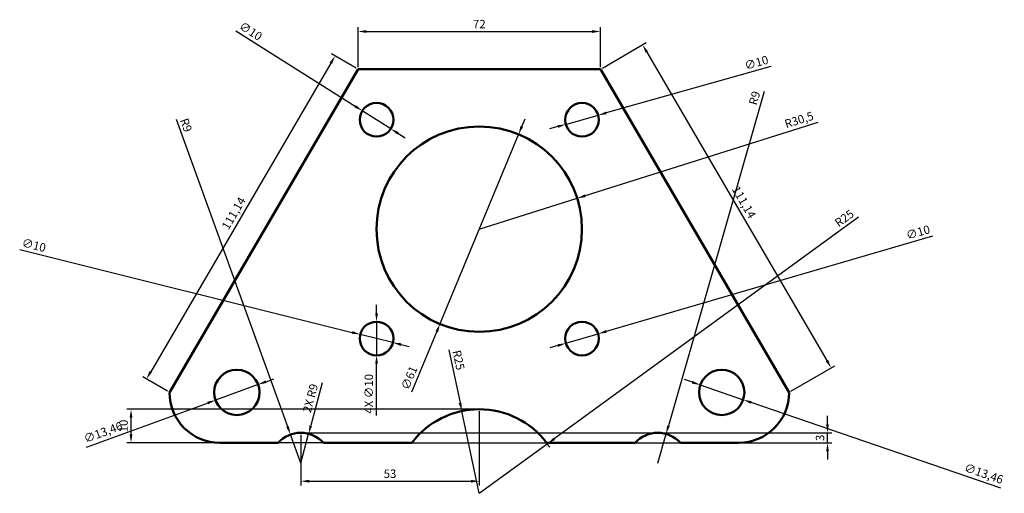
# Model space of a CAD drawing. Units: millimetres. Extents: x 120 to 412, y 203 to 344.
import ezdxf

# ---------------------------------------------------------------- set-up
doc = ezdxf.new("R2010")
doc.units = ezdxf.units.MM
doc.layers.add('M-DIMS', color=2, linetype='Continuous', lineweight=25)
doc.layers.add('M-OUTL', color=7, linetype='Continuous', lineweight=50)
doc.styles.get("Standard").update_dxf_attribs({"font": 'arial.ttf'})
doc.dimstyles.new('ISO-25', dxfattribs={"dimtxt": 2.5, "dimasz": 2.5, "dimexe": 1.25, "dimexo": 0.625, "dimtad": 1, "dimtxsty": 'Standard', "dimcen": 2.5, "dimadec": 0, "dimazin": 0, "dimtfac": 1, "dimtmove": 0, "dimatfit": 3, "dimfxl": 1, "dimarcsym": 0})

# ---------------------------------------------------------------- blocks, each defined once
blk = doc.blocks.new('*D1')
at = {"layer": 'Defpoints', "color": 0, "transparency": 16777216}
for p in [(292.1, 328.85), (360.58, 240.13), (348.1, 232.85)]:
    blk.add_point(p, dxfattribs=at)
at = {"layer": 'M-DIMS', "color": 0, "lineweight": -2, "transparency": 16777216}
for p, q in [((292.64, 329.16), (305.66, 336.76)), ((305.84, 333.97), (359.32, 242.29)), ((348.64, 233.16), (361.66, 240.76))]:
    blk.add_line(p, q, dxfattribs=at)
at = {"layer": 'M-DIMS', "color": 0, "transparency": 16777216}
for points in [[(306.2, 334.18), (305.48, 333.76), (304.58, 336.13)], [(359.68, 242.5), (358.96, 242.08), (360.58, 240.13)]]:
    blk.add_solid(points, dxfattribs=at)
at = {"layer": 'M-DIMS', "color": 0, "transparency": 16777216, "insert": (334.42, 289.2), "char_height": 2.5, "attachment_point": 5, "rotation": 300.2564}
blk.add_mtext('111,14', dxfattribs=at)
blk = doc.blocks.new('*D2')
at = {"layer": 'Defpoints', "color": 0, "transparency": 16777216}
for p in [(292.1, 340.07), (220.1, 328.85), (292.1, 328.85)]:
    blk.add_point(p, dxfattribs=at)
at = {"layer": 'M-DIMS', "color": 0, "lineweight": -2, "transparency": 16777216}
for p, q in [((220.1, 329.47), (220.1, 341.32)), ((222.6, 340.07), (289.6, 340.07)), ((292.1, 329.47), (292.1, 341.32))]:
    blk.add_line(p, q, dxfattribs=at)
at = {"layer": 'M-DIMS', "color": 0, "transparency": 16777216}
for points in [[(222.6, 340.49), (222.6, 339.65), (220.1, 340.07)], [(289.6, 340.49), (289.6, 339.65), (292.1, 340.07)]]:
    blk.add_solid(points, dxfattribs=at)
at = {"layer": 'M-DIMS', "color": 0, "transparency": 16777216, "insert": (256.1, 341.95), "char_height": 2.5, "attachment_point": 5}
blk.add_mtext('72', dxfattribs=at)
blk = doc.blocks.new('*D3')
at = {"layer": 'Defpoints', "color": 0, "transparency": 16777216}
for p in [(220.1, 328.85), (157.28, 236.82), (164.1, 232.85)]:
    blk.add_point(p, dxfattribs=at)
at = {"layer": 'M-DIMS', "color": 0, "lineweight": -2, "transparency": 16777216}
for p, q in [((219.56, 329.16), (212.2, 333.45)), ((212.02, 330.66), (158.54, 238.98)), ((163.56, 233.16), (156.2, 237.45))]:
    blk.add_line(p, q, dxfattribs=at)
at = {"layer": 'M-DIMS', "color": 0, "transparency": 16777216}
for points in [[(211.66, 330.87), (212.38, 330.45), (213.28, 332.82)], [(158.18, 239.19), (158.9, 238.77), (157.28, 236.82)]]:
    blk.add_solid(points, dxfattribs=at)
at = {"layer": 'M-DIMS', "color": 0, "transparency": 16777216, "insert": (183.45, 285.89), "char_height": 2.5, "attachment_point": 5, "rotation": 59.7436}
blk.add_mtext('111,14', dxfattribs=at)
blk = doc.blocks.new('*D4')
at = {"layer": 'Defpoints', "color": 0, "transparency": 16777216}
for p in [(200.03, 220.31), (203.1, 211.85)]:
    blk.add_point(p, dxfattribs=at)
at = {"layer": 'M-DIMS', "color": 0, "lineweight": -2, "transparency": 16777216}
for p, q in [((166.06, 313.98), (199.18, 222.66)), ((203.1, 211.85), (200.03, 220.31))]:
    blk.add_line(p, q, dxfattribs=at)
at = {"layer": 'M-DIMS', "color": 0, "transparency": 16777216}
blk.add_solid([(199.57, 222.8), (198.79, 222.52), (200.03, 220.31)], dxfattribs=at)
at = {"layer": 'M-DIMS', "color": 0, "transparency": 16777216, "insert": (168.75, 312.14), "char_height": 2.5, "attachment_point": 5, "rotation": 289.9316}
blk.add_mtext('R9', dxfattribs=at)
blk = doc.blocks.new('*D5')
at = {"layer": 'Defpoints', "color": 0, "transparency": 16777216}
for p in [(311.57, 220.5), (309.1, 211.85)]:
    blk.add_point(p, dxfattribs=at)
at = {"layer": 'M-DIMS', "color": 0, "lineweight": -2, "transparency": 16777216}
for p, q in [((340.7, 322.23), (312.26, 222.9)), ((309.1, 211.85), (311.57, 220.5))]:
    blk.add_line(p, q, dxfattribs=at)
at = {"layer": 'M-DIMS', "color": 0, "transparency": 16777216}
blk.add_solid([(311.86, 223.02), (312.66, 222.79), (311.57, 220.5)], dxfattribs=at)
at = {"layer": 'M-DIMS', "color": 0, "transparency": 16777216, "insert": (338.14, 320.21), "char_height": 2.5, "attachment_point": 5, "rotation": 74.0249}
blk.add_mtext('R9', dxfattribs=at)
blk = doc.blocks.new('*D6')
at = {"layer": 'Defpoints', "color": 0, "transparency": 16777216}
for p in [(276.3, 217.57), (256.1, 202.85)]:
    blk.add_point(p, dxfattribs=at)
at = {"layer": 'M-DIMS', "color": 0, "lineweight": -2, "transparency": 16777216}
for p, q in [((368.71, 284.93), (278.32, 219.05)), ((256.1, 202.85), (276.3, 217.57))]:
    blk.add_line(p, q, dxfattribs=at)
blk.add_arc((256.1, 202.85), 25, 33.2231, 36.8699, dxfattribs=at)
at = {"layer": 'M-DIMS', "color": 0, "transparency": 16777216}
blk.add_solid([(278.08, 219.38), (278.57, 218.71), (276.3, 217.57)], dxfattribs=at)
at = {"layer": 'M-DIMS', "color": 0, "transparency": 16777216, "insert": (364.67, 284.34), "char_height": 2.5, "attachment_point": 5, "rotation": 36.0879}
blk.add_mtext('R25', dxfattribs=at)
blk = doc.blocks.new('*D7')
at = {"layer": 'Defpoints', "color": 0, "transparency": 16777216}
for p in [(285.19, 290.51), (256.1, 281.35)]:
    blk.add_point(p, dxfattribs=at)
at = {"layer": 'M-DIMS', "color": 0, "lineweight": -2, "transparency": 16777216}
for p, q in [((356.64, 313.02), (287.57, 291.26)), ((256.1, 281.35), (285.19, 290.51))]:
    blk.add_line(p, q, dxfattribs=at)
at = {"layer": 'M-DIMS', "color": 0, "transparency": 16777216}
blk.add_solid([(287.45, 291.66), (287.7, 290.87), (285.19, 290.51)], dxfattribs=at)
at = {"layer": 'M-DIMS', "color": 0, "transparency": 16777216, "insert": (351.15, 313.52), "char_height": 2.5, "attachment_point": 5, "rotation": 17.4843}
blk.add_mtext('R30,5', dxfattribs=at)
blk = doc.blocks.new('*D8')
at = {"layer": 'Defpoints', "color": 0, "transparency": 16777216}
for p in [(291.41, 315.2), (281.78, 312.49)]:
    blk.add_point(p, dxfattribs=at)
at = {"layer": 'M-DIMS', "color": 0, "lineweight": -2, "transparency": 16777216}
for p, q in [((342.63, 329.63), (293.82, 315.88)), ((281.78, 312.49), (291.41, 315.2)), ((279.38, 311.81), (276.97, 311.14))]:
    blk.add_line(p, q, dxfattribs=at)
at = {"layer": 'M-DIMS', "color": 0, "transparency": 16777216}
for points in [[(293.7, 316.28), (293.93, 315.48), (291.41, 315.2)], [(279.27, 312.22), (279.49, 311.41), (281.78, 312.49)]]:
    blk.add_solid(points, dxfattribs=at)
at = {"layer": 'M-DIMS', "color": 0, "transparency": 16777216, "insert": (338.47, 330.51), "char_height": 2.5, "attachment_point": 5, "rotation": 15.7318}
blk.add_mtext('∅10', dxfattribs=at)
blk = doc.blocks.new('*D9')
at = {"layer": 'Defpoints', "color": 0, "transparency": 16777216}
for p in [(221.37, 316.52), (229.82, 311.18)]:
    blk.add_point(p, dxfattribs=at)
at = {"layer": 'M-DIMS', "color": 0, "lineweight": -2, "transparency": 16777216}
for p, q in [((183.8, 340.27), (219.26, 317.86)), ((229.82, 311.18), (221.37, 316.52)), ((231.94, 309.84), (234.05, 308.5))]:
    blk.add_line(p, q, dxfattribs=at)
at = {"layer": 'M-DIMS', "color": 0, "transparency": 16777216}
for points in [[(219.48, 318.21), (219.04, 317.5), (221.37, 316.52)], [(232.16, 310.19), (231.71, 309.49), (229.82, 311.18)]]:
    blk.add_solid(points, dxfattribs=at)
at = {"layer": 'M-DIMS', "color": 0, "transparency": 16777216, "insert": (188.05, 339.92), "char_height": 2.5, "attachment_point": 5, "rotation": 327.6988}
blk.add_mtext('∅10', dxfattribs=at)
blk = doc.blocks.new('*D10')
at = {"layer": 'Defpoints', "color": 0, "transparency": 16777216}
for p in [(220.75, 250.06), (230.45, 247.64)]:
    blk.add_point(p, dxfattribs=at)
at = {"layer": 'M-DIMS', "color": 0, "lineweight": -2, "transparency": 16777216}
for p, q in [((119.63, 275.27), (218.32, 250.66)), ((230.45, 247.64), (220.75, 250.06)), ((232.87, 247.03), (235.3, 246.43))]:
    blk.add_line(p, q, dxfattribs=at)
at = {"layer": 'M-DIMS', "color": 0, "transparency": 16777216}
for points in [[(218.42, 251.07), (218.22, 250.26), (220.75, 250.06)], [(232.98, 247.44), (232.77, 246.63), (230.45, 247.64)]]:
    blk.add_solid(points, dxfattribs=at)
at = {"layer": 'M-DIMS', "color": 0, "transparency": 16777216, "insert": (123.77, 276.27), "char_height": 2.5, "attachment_point": 5, "rotation": 345.9971}
blk.add_mtext('∅10', dxfattribs=at)
blk = doc.blocks.new('*D11')
at = {"layer": 'Defpoints', "color": 0, "transparency": 16777216}
for p in [(291.4, 250.25), (281.8, 247.44)]:
    blk.add_point(p, dxfattribs=at)
at = {"layer": 'M-DIMS', "color": 0, "lineweight": -2, "transparency": 16777216}
for p, q in [((390.64, 279.28), (293.8, 250.95)), ((281.8, 247.44), (291.4, 250.25)), ((279.4, 246.74), (277, 246.04))]:
    blk.add_line(p, q, dxfattribs=at)
at = {"layer": 'M-DIMS', "color": 0, "transparency": 16777216}
for points in [[(293.68, 251.35), (293.91, 250.55), (291.4, 250.25)], [(279.28, 247.14), (279.52, 246.34), (281.8, 247.44)]]:
    blk.add_solid(points, dxfattribs=at)
at = {"layer": 'M-DIMS', "color": 0, "transparency": 16777216, "insert": (386.47, 280.11), "char_height": 2.5, "attachment_point": 5, "rotation": 16.3027}
blk.add_mtext('∅10', dxfattribs=at)
blk = doc.blocks.new('*D12')
at = {"layer": 'Defpoints', "color": 0, "transparency": 16777216}
for p in [(321.73, 235.04), (334.46, 230.66)]:
    blk.add_point(p, dxfattribs=at)
at = {"layer": 'M-DIMS', "color": 0, "lineweight": -2, "transparency": 16777216}
for p, q in [((319.37, 235.85), (317.01, 236.66)), ((321.73, 235.04), (334.46, 230.66)), ((410.98, 204.35), (336.82, 229.85))]:
    blk.add_line(p, q, dxfattribs=at)
at = {"layer": 'M-DIMS', "color": 0, "transparency": 16777216}
for points in [[(319.51, 236.24), (319.23, 235.45), (321.73, 235.04)], [(336.96, 230.24), (336.69, 229.45), (334.46, 230.66)]]:
    blk.add_solid(points, dxfattribs=at)
at = {"layer": 'M-DIMS', "color": 0, "transparency": 16777216, "insert": (405.82, 208.42), "char_height": 2.5, "attachment_point": 5, "rotation": 341.0278}
blk.add_mtext('∅13,46', dxfattribs=at)
blk = doc.blocks.new('*D13')
at = {"layer": 'Defpoints', "color": 0, "transparency": 16777216}
for p in [(190.42, 235.16), (177.78, 230.54)]:
    blk.add_point(p, dxfattribs=at)
at = {"layer": 'M-DIMS', "color": 0, "lineweight": -2, "transparency": 16777216}
for p, q in [((192.77, 236.01), (195.11, 236.87)), ((190.42, 235.16), (177.78, 230.54)), ((139.42, 216.54), (175.43, 229.68))]:
    blk.add_line(p, q, dxfattribs=at)
at = {"layer": 'M-DIMS', "color": 0, "transparency": 16777216}
for points in [[(192.62, 236.4), (192.91, 235.62), (190.42, 235.16)], [(175.29, 230.07), (175.57, 229.29), (177.78, 230.54)]]:
    blk.add_solid(points, dxfattribs=at)
at = {"layer": 'M-DIMS', "color": 0, "transparency": 16777216, "insert": (144.5, 220.7), "char_height": 2.5, "attachment_point": 5, "rotation": 20.0551}
blk.add_mtext('∅13,46', dxfattribs=at)
blk = doc.blocks.new('MOUNT-HOLE-D10')
blk.add_circle((5, 5), 5)
blk = doc.blocks.new('FLANGE-MOUNT-HOLE')
blk.add_circle((6.73, 6.73), 6.73)
blk = doc.blocks.new('*D16')
at = {"layer": 'Defpoints', "color": 0, "transparency": 16777216}
for p in [(203.1, 220.85), (359.5, 220.85), (209.81, 217.85)]:
    blk.add_point(p, dxfattribs=at)
at = {"layer": 'M-DIMS', "color": 0, "lineweight": -2, "transparency": 16777216}
for p, q in [((359.5, 223.35), (359.5, 225.85)), ((203.72, 220.85), (360.75, 220.85)), ((359.5, 217.85), (359.5, 220.85)), ((210.43, 217.85), (360.75, 217.85)), ((359.5, 215.35), (359.5, 212.85))]:
    blk.add_line(p, q, dxfattribs=at)
at = {"layer": 'M-DIMS', "color": 0, "transparency": 16777216}
for points in [[(359.08, 223.35), (359.91, 223.35), (359.5, 220.85)], [(359.08, 215.35), (359.91, 215.35), (359.5, 217.85)]]:
    blk.add_solid(points, dxfattribs=at)
at = {"layer": 'M-DIMS', "color": 0, "transparency": 16777216, "insert": (357.6, 219.35), "char_height": 2.5, "attachment_point": 5, "rotation": 90}
blk.add_mtext('3', dxfattribs=at)
blk = doc.blocks.new('*D17')
at = {"layer": 'Defpoints', "color": 0, "transparency": 16777216}
for p in [(152.7, 227.85), (256.1, 227.85), (236.1, 217.85)]:
    blk.add_point(p, dxfattribs=at)
at = {"layer": 'M-DIMS', "color": 0, "lineweight": -2, "transparency": 16777216}
for p, q in [((255.47, 227.85), (151.45, 227.85)), ((152.7, 220.35), (152.7, 225.35)), ((235.47, 217.85), (151.45, 217.85))]:
    blk.add_line(p, q, dxfattribs=at)
at = {"layer": 'M-DIMS', "color": 0, "transparency": 16777216}
for points in [[(152.28, 225.35), (153.11, 225.35), (152.7, 227.85)], [(152.28, 220.35), (153.11, 220.35), (152.7, 217.85)]]:
    blk.add_solid(points, dxfattribs=at)
at = {"layer": 'M-DIMS', "color": 0, "transparency": 16777216, "insert": (150.8, 222.85), "char_height": 2.5, "attachment_point": 5, "rotation": 90}
blk.add_mtext('10', dxfattribs=at)
blk = doc.blocks.new('*D18')
at = {"layer": 'Defpoints', "color": 0, "transparency": 16777216}
for p in [(256.1, 227.85), (203.1, 220.85), (256.1, 206.45)]:
    blk.add_point(p, dxfattribs=at)
at = {"layer": 'M-DIMS', "color": 0, "lineweight": -2, "transparency": 16777216}
for p, q in [((256.1, 227.22), (256.1, 205.2)), ((203.1, 220.22), (203.1, 205.2)), ((205.6, 206.45), (253.6, 206.45))]:
    blk.add_line(p, q, dxfattribs=at)
at = {"layer": 'M-DIMS', "color": 0, "transparency": 16777216}
for points in [[(205.6, 206.86), (205.6, 206.03), (203.1, 206.45)], [(253.6, 206.86), (253.6, 206.03), (256.1, 206.45)]]:
    blk.add_solid(points, dxfattribs=at)
at = {"layer": 'M-DIMS', "color": 0, "transparency": 16777216, "insert": (229.6, 208.35), "char_height": 2.5, "attachment_point": 5}
blk.add_mtext('53', dxfattribs=at)
blk = doc.blocks.new('*D19')
at = {"layer": 'Defpoints', "color": 0, "transparency": 16777216}
for p in [(267.77, 309.53), (244.43, 253.17)]:
    blk.add_point(p, dxfattribs=at)
at = {"layer": 'M-DIMS', "color": 0, "lineweight": -2, "transparency": 16777216}
for p, q in [((268.73, 311.84), (269.68, 314.15)), ((267.77, 309.53), (244.43, 253.17)), ((236.07, 233), (243.47, 250.86))]:
    blk.add_line(p, q, dxfattribs=at)
at = {"layer": 'M-DIMS', "color": 0, "transparency": 16777216}
for points in [[(268.34, 312), (269.11, 311.68), (267.77, 309.53)], [(243.08, 251.02), (243.85, 250.7), (244.43, 253.17)]]:
    blk.add_solid(points, dxfattribs=at)
at = {"layer": 'M-DIMS', "color": 0, "transparency": 16777216, "insert": (235.6, 237.02), "char_height": 2.5, "attachment_point": 5, "rotation": 67.4992}
blk.add_mtext('∅61', dxfattribs=at)
blk = doc.blocks.new('*D20')
at = {"layer": 'Defpoints', "color": 0, "transparency": 16777216}
for p in [(225.6, 253.85), (225.6, 243.85)]:
    blk.add_point(p, dxfattribs=at)
at = {"layer": 'M-DIMS', "color": 0, "lineweight": -2, "transparency": 16777216}
for p, q in [((225.6, 256.35), (225.6, 258.85)), ((225.6, 253.85), (225.6, 243.85)), ((225.6, 225.97), (225.6, 241.35))]:
    blk.add_line(p, q, dxfattribs=at)
at = {"layer": 'M-DIMS', "color": 0, "transparency": 16777216}
for points in [[(225.18, 256.35), (226.01, 256.35), (225.6, 253.85)], [(225.18, 241.35), (226.01, 241.35), (225.6, 243.85)]]:
    blk.add_solid(points, dxfattribs=at)
at = {"layer": 'M-DIMS', "color": 0, "transparency": 16777216, "insert": (223.62, 232.41), "char_height": 2.5, "attachment_point": 5, "rotation": 89.9966}
blk.add_mtext('4X ∅10', dxfattribs=at)
blk = doc.blocks.new('*D21')
at = {"layer": 'Defpoints', "color": 0, "transparency": 16777216}
for p in [(205.43, 220.54), (203.1, 211.85)]:
    blk.add_point(p, dxfattribs=at)
at = {"layer": 'M-DIMS', "color": 0, "lineweight": -2, "transparency": 16777216}
for p, q in [((209.49, 235.71), (206.07, 222.96)), ((203.1, 211.85), (205.43, 220.54))]:
    blk.add_line(p, q, dxfattribs=at)
at = {"layer": 'M-DIMS', "color": 0, "transparency": 16777216}
blk.add_solid([(205.67, 223.06), (206.48, 222.85), (205.43, 220.54)], dxfattribs=at)
at = {"layer": 'M-DIMS', "color": 0, "transparency": 16777216, "insert": (206.27, 231.03), "char_height": 2.5, "attachment_point": 5, "rotation": 75.0031}
blk.add_mtext('2X R9', dxfattribs=at)
blk = doc.blocks.new('*D22')
at = {"layer": 'Defpoints', "color": 0, "transparency": 16777216}
for p in [(250.9, 227.3), (256.1, 202.85)]:
    blk.add_point(p, dxfattribs=at)
at = {"layer": 'M-DIMS', "color": 0, "lineweight": -2, "transparency": 16777216}
for p, q in [((247.03, 245.52), (250.38, 229.75)), ((256.1, 202.85), (250.9, 227.3))]:
    blk.add_line(p, q, dxfattribs=at)
at = {"layer": 'M-DIMS', "color": 0, "transparency": 16777216}
blk.add_solid([(250.79, 229.83), (249.97, 229.66), (250.9, 227.3)], dxfattribs=at)
at = {"layer": 'M-DIMS', "color": 0, "transparency": 16777216, "insert": (249.64, 242.37), "char_height": 2.5, "attachment_point": 5, "rotation": 282.0011}
blk.add_mtext('R25', dxfattribs=at)

msp = doc.modelspace()

# ---------------------------------------------------------------- linework, layer by layer
at = {"layer": 'M-OUTL'}
for p, q in [((220.097, 328.848), (164.097, 232.848)), ((256.097, 328.848), (220.097, 328.848)), ((256.097, 328.848), (292.097, 328.848)), ((292.097, 328.848), (348.097, 232.848)), ((164.097, 232.848), (164.097, 232.848)), ((348.097, 232.848), (348.097, 232.848)), ((196.389, 217.848), (179.097, 217.848)), ((236.097, 217.848), (209.806, 217.848)), ((276.097, 217.848), (302.389, 217.848)), ((315.806, 217.848), (333.097, 217.848))]:
    msp.add_line(p, q, dxfattribs=at)
msp.add_circle((256.097, 281.348), 30.5, dxfattribs=at)
for centre, radius, start, end in [((179.097, 232.848), 15, 180, 270), ((333.097, 232.848), 15, 270, 0), ((256.097, 202.848), 25, 36.8699, 143.1301), ((203.097, 211.848), 9, 41.81031, 138.18969), ((309.097, 211.848), 9, 41.81031, 138.18969)]:
    msp.add_arc(centre, radius, start, end, dxfattribs=at)

# ---------------------------------------------------------------- block references
for name, p in [('MOUNT-HOLE-D10', (220.597, 308.848)), ('MOUNT-HOLE-D10', (281.597, 308.848)), ('MOUNT-HOLE-D10', (220.597, 243.848)), ('MOUNT-HOLE-D10', (281.597, 243.848)), ('FLANGE-MOUNT-HOLE', (177.368, 226.119)), ('FLANGE-MOUNT-HOLE', (321.368, 226.119))]:
    msp.add_blockref(name, p, dxfattribs=at)

# ---------------------------------------------------------------- dimensions: what is measured, and where the dimension line sits
at = {"layer": 'M-DIMS'}
for p1, p2, override, picture, middle in [((229.824, 311.176), (221.371, 316.52), {"dimclrd": 0, "dimclre": 0, "dimclrt": 0}, '*D9', (186.992, 338.255)), ((281.785, 312.493), (291.41, 315.204), {"dimclrd": 0, "dimclre": 0, "dimclrt": 0}, '*D8', (339.005, 328.611)), ((267.77, 309.526), (244.425, 253.17), {"dimdec": 0, "dimlfac": 1, "dimrnd": 0, "dimzin": 0, "dimdsep": 46, "dimlunit": 2}, '*D19', (237.422, 236.263)), ((281.798, 247.445), (291.396, 250.252), {"dimclrd": 0, "dimclre": 0, "dimclrt": 0}, '*D11', (387.021, 278.219)), ((230.449, 247.638), (220.746, 250.058), {"dimclrd": 0, "dimclre": 0, "dimclrt": 0}, '*D10', (123.291, 274.362)), ((190.418, 235.156), (177.776, 230.541), {"dimclrd": 0, "dimclre": 0, "dimclrt": 0}, '*D13', (145.248, 218.666)), ((321.734, 235.036), (334.461, 230.661), {"dimclrd": 0, "dimclre": 0, "dimclrt": 0}, '*D12', (405.118, 206.37))]:
    dim = msp.add_diameter_dim_2p(p1=p1, p2=p2, dimstyle='ISO-25', override=override, dxfattribs=at)
    dim.commit()
    dim.dimension.update_dxf_attribs({"geometry": picture, "text_midpoint": middle, "dimtype": 163})
for base, p1, p2, override, picture, middle in [((292.097, 340.069), (220.097, 328.848), (292.097, 328.848), {"dimclrd": 0, "dimclre": 0, "dimclrt": 0}, '*D2', (256.097, 341.949)), ((256.097, 206.448), (203.097, 220.848), (256.097, 227.848), {"dimdec": 0, "dimlfac": 1, "dimrnd": 0, "dimzin": 0, "dimdsep": 46, "dimlunit": 2}, '*D18', (229.597, 208.351))]:
    dim = msp.add_linear_dim(base=base, p1=p1, p2=p2, dimstyle='ISO-25', override=override, dxfattribs=at)
    dim.commit()
    dim.dimension.update_dxf_attribs({"geometry": picture, "text_midpoint": middle})
for p1, p2, distance, picture, middle in [((292.097, 328.848), (348.097, 232.848), 14.453, '*D1', (334.419, 289.203)), ((220.097, 328.848), (164.097, 232.848), -7.888, '*D3', (183.446, 285.895))]:
    dim = msp.add_aligned_dim(p1=p1, p2=p2, distance=distance, dimstyle='ISO-25', override={"dimclrd": 0, "dimclre": 0, "dimclrt": 0}, dxfattribs=at)
    dim.commit()
    dim.dimension.update_dxf_attribs({"geometry": picture, "text_midpoint": middle})
for center, mpoint, override, picture, middle in [((309.097, 211.848), (311.574, 220.501), {"dimclrd": 0, "dimclre": 0, "dimclrt": 0}, '*D5', (339.97, 319.69)), ((256.097, 281.348), (285.188, 290.512), {"dimclrd": 0, "dimclre": 0, "dimclrt": 0}, '*D7', (351.793, 311.492)), ((203.097, 211.848), (200.029, 220.309), {"dimclrd": 0, "dimclre": 0, "dimclrt": 0}, '*D4', (166.964, 311.492)), ((256.097, 202.848), (276.3, 217.574), {"dimclrd": 0, "dimclre": 0, "dimclrt": 0}, '*D6', (365.788, 282.8)), ((256.097, 202.848), (250.899, 227.302), {"dimdec": 0, "dimlfac": 1, "dimrnd": 0, "dimzin": 0, "dimdsep": 46, "dimlunit": 2}, '*D22', (247.78, 241.974))]:
    dim = msp.add_radius_dim(center=center, mpoint=mpoint, dimstyle='ISO-25', override=override, dxfattribs=at)
    dim.commit()
    dim.dimension.update_dxf_attribs({"geometry": picture, "text_midpoint": middle, "dimtype": 164})
dim = msp.add_diameter_dim_2p(p1=(225.598, 253.848), p2=(225.597, 243.848), text='4X <>', dimstyle='ISO-25', override={"dimdec": 0, "dimlfac": 1, "dimrnd": 0, "dimzin": 0, "dimdsep": 46, "dimlunit": 2}, dxfattribs=at)
dim.commit()
dim.dimension.update_dxf_attribs({"geometry": '*D20', "text_midpoint": (225.596, 232.407), "dimtype": 163})
dim = msp.add_radius_dim(center=(203.097, 211.848), mpoint=(205.426, 220.542), text='2X <>', dimstyle='ISO-25', override={"dimdec": 0, "dimlfac": 1, "dimrnd": 0, "dimzin": 0, "dimdsep": 46, "dimlunit": 2}, dxfattribs=at)
dim.commit()
dim.dimension.update_dxf_attribs({"geometry": '*D21', "text_midpoint": (206.268, 231.032)})
for base, p1, p2, picture, middle in [((152.697, 227.848), (236.097, 217.848), (256.097, 227.848), '*D17', (150.796, 222.848)), ((359.497, 220.848), (209.806, 217.848), (203.097, 220.848), '*D16', (357.595, 219.348))]:
    dim = msp.add_linear_dim(base=base, p1=p1, p2=p2, angle=90, dimstyle='ISO-25', override={"dimdec": 0, "dimlfac": 1, "dimrnd": 0, "dimzin": 0, "dimdsep": 46, "dimlunit": 2}, dxfattribs=at)
    dim.commit()
    dim.dimension.update_dxf_attribs({"geometry": picture, "text_midpoint": middle})

doc.saveas('drawing.dxf')
